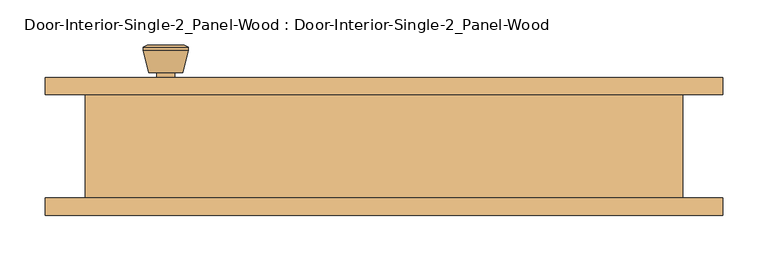
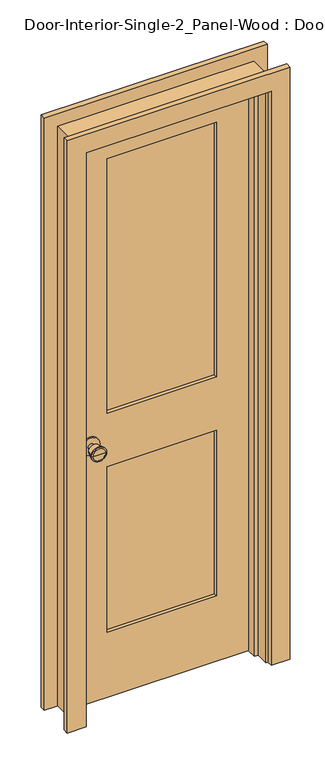
"""IFC4 building model written with IfcOpenShell, lengths in millimetres: door geometry, Door-Interior-Single-2_Panel-Wood : Door-Interior-Single-2_Panel-Wood."""

from ifc_helpers import new_model, si_unit, point, frame, frame_2d, origin, place, context, project, spatial, polyline, circle_curve, trimmed, segment, composite_curve, outline, extrude, faceted_brep, source, transform, mapped, element, save
from ifc_brep_helpers import plane_surface, cylinder_surface, revolved_surface, advanced_brep


def door_interior_single_2_panel_wood_door_interior_single_2_a051e6ed(model_context):
    return source(origin(), model_context, "Body", "SolidModel", [
        advanced_brep(
        [(-241.3, 13.05, 914.4), (-231.3, 13.05, 914.4), (-251.3, 13.05, 914.4), (-220.8241324, -35.95, 914.4), (-241.3, -35.95, 914.4), (-261.7758676, -35.95, 914.4), (-216.3, -34.1221319, 914.4), (-266.3, -34.1221319, 914.4), (-216.3, -30.6584537, 914.4), (-266.3, -30.6584537, 914.4), (-222.663764, -5.95, 914.4), (-259.936236, -5.95, 914.4), (-231.3, -5.95, 914.4), (-251.3, -5.95, 914.4)],
        [
            (0, 1),
            (1, 2, circle_curve(frame((-241.3, 13.05, 914.4), z_axis=(0.0, 1.0, 0.0), x_axis=(-1.0, 0.0, 0.0)), 10.0)),
            (2, 0),
            (2, 1, circle_curve(frame((-241.3, 13.05, 914.4), z_axis=(0.0, 1.0, 0.0), x_axis=(-1.0, 0.0, 0.0)), 10.0)),
            (3, 4),
            (4, 5),
            (5, 3, circle_curve(frame((-241.3, -35.95, 914.4), z_axis=(0.0, -1.0, 0.0), x_axis=(-1.0, 0.0, 0.0)), 20.4758676)),
            (3, 5, circle_curve(frame((-241.3, -35.95, 914.4), z_axis=(0.0, -1.0, 0.0), x_axis=(-1.0, 0.0, 0.0)), 20.4758676)),
            (6, 3),
            (5, 7),
            (7, 6, circle_curve(frame((-241.3, -34.1221319, 914.4), z_axis=(0.0, -1.0, 0.0), x_axis=(-1.0, 0.0, 0.0)), 25.0)),
            (6, 7, circle_curve(frame((-241.3, -34.1221319, 914.4), z_axis=(0.0, -1.0, 0.0), x_axis=(-1.0, 0.0, 0.0)), 25.0)),
            (8, 6),
            (7, 9),
            (9, 8, circle_curve(frame((-241.3, -30.6584537, 914.4), z_axis=(0.0, -1.0, 0.0), x_axis=(-1.0, 0.0, 0.0)), 25.0)),
            (8, 9, circle_curve(frame((-241.3, -30.6584537, 914.4), z_axis=(0.0, -1.0, 0.0), x_axis=(-1.0, 0.0, 0.0)), 25.0)),
            (10, 8),
            (9, 11),
            (11, 10, circle_curve(frame((-241.3, -5.95, 914.4), z_axis=(0.0, -1.0, 0.0), x_axis=(-1.0, 0.0, 0.0)), 18.636236)),
            (10, 11, circle_curve(frame((-241.3, -5.95, 914.4), z_axis=(0.0, -1.0, 0.0), x_axis=(-1.0, 0.0, 0.0)), 18.636236)),
            (12, 10),
            (11, 13),
            (13, 12, circle_curve(frame((-241.3, -5.95, 914.4), z_axis=(0.0, -1.0, 0.0), x_axis=(-1.0, 0.0, 0.0)), 10.0)),
            (12, 13, circle_curve(frame((-241.3, -5.95, 914.4), z_axis=(0.0, -1.0, 0.0), x_axis=(-1.0, 0.0, 0.0)), 10.0)),
            (1, 12),
            (13, 2),
        ],
        [
            plane_surface(frame((-241.3, 13.05, 914.4), z_axis=(0.0, 1.0, 0.0), x_axis=(-1.0, 0.0, 0.0))),
            plane_surface(frame((-241.3, -35.95, 914.4), z_axis=(0.0, -1.0, 0.0), x_axis=(-1.0, 0.0, 0.0))),
            revolved_surface(polyline([(-261.7758676, -35.95, 914.4), (-266.3, -34.1221319, 914.4)]), (-241.3, 13.05, 914.4), (0.0, 1.0, 0.0)),
            cylinder_surface(frame((-241.3, 13.05, 914.4), z_axis=(0.0, 1.0, 0.0), x_axis=(-1.0, 0.0, 0.0)), 25.0),
            revolved_surface(polyline([(-266.3, -30.6584537, 914.4), (-259.936236, -5.95, 914.4)]), (-241.3, 13.05, 914.4), (0.0, 1.0, 0.0)),
            plane_surface(frame((-241.3, -5.95, 914.4), z_axis=(0.0, 1.0, 0.0), x_axis=(-1.0, 0.0, 0.0))),
            cylinder_surface(frame((-241.3, 13.05, 914.4), z_axis=(0.0, 1.0, 0.0), x_axis=(-1.0, 0.0, 0.0)), 10.0),
        ],
        [
            (0, [[1, 2, 3]]),
            (0, [[-3, 4, -1]]),
            (1, [[5, 6, 7]]),
            (1, [[-6, -5, 8]]),
            (2, [[9, -7, 10, 11]]),
            (2, [[-10, -8, -9, 12]]),
            (3, [[13, -11, 14, 15]]),
            (3, [[-14, -12, -13, 16]]),
            (4, [[17, -15, 18, 19]]),
            (4, [[-18, -16, -17, 20]]),
            (5, [[21, -19, 22, 23]]),
            (5, [[-22, -20, -21, 24]]),
            (6, [[25, -23, 26, -2]]),
            (6, [[-26, -24, -25, -4]]),
        ],
    ),
        extrude(outline(composite_curve([segment(trimmed(circle_curve(frame_2d((914.4, -241.3)), 30.0), [point((914.4, -271.3))], [point((914.4, -211.3))], False, "CARTESIAN"), True, "CONTINUOUS"), segment(trimmed(circle_curve(frame_2d((914.4, -241.3)), 30.0), [point((914.4, -211.3))], [point((914.4, -271.3))], False, "CARTESIAN"), True, "CONTINUOUS")], self_intersect=False)), frame((0.0, 13.05, 0.0), z_axis=(0.0, 1.0, 0.0), x_axis=(0.0, 0.0, 1.0)), (0.0, 0.0, 1.0), 6.0),
        advanced_brep(
        [(-241.3, 59.975, 914.4), (-251.3, 59.975, 914.4), (-231.3, 59.975, 914.4), (-220.8241324, 108.975, 914.4), (-261.7758676, 108.975, 914.4), (-241.3, 108.975, 914.4), (-216.3, 107.1471319, 914.4), (-266.3, 107.1471319, 914.4), (-216.3, 103.6834537, 914.4), (-266.3, 103.6834537, 914.4), (-222.663764, 78.975, 914.4), (-259.936236, 78.975, 914.4), (-231.3, 78.975, 914.4), (-251.3, 78.975, 914.4)],
        [
            (0, 1),
            (1, 2, circle_curve(frame((-241.3, 59.975, 914.4), z_axis=(0.0, -1.0, 0.0), x_axis=(-1.0, 0.0, 0.0)), 10.0)),
            (2, 0),
            (2, 1, circle_curve(frame((-241.3, 59.975, 914.4), z_axis=(0.0, -1.0, 0.0), x_axis=(-1.0, 0.0, 0.0)), 10.0)),
            (3, 4, circle_curve(frame((-241.3, 108.975, 914.4), z_axis=(0.0, 1.0, 0.0), x_axis=(-1.0, 0.0, 0.0)), 20.4758676)),
            (4, 5),
            (5, 3),
            (4, 3, circle_curve(frame((-241.3, 108.975, 914.4), z_axis=(0.0, 1.0, 0.0), x_axis=(-1.0, 0.0, 0.0)), 20.4758676)),
            (6, 7, circle_curve(frame((-241.3, 107.1471319, 914.4), z_axis=(0.0, 1.0, 0.0), x_axis=(-1.0, 0.0, 0.0)), 25.0)),
            (7, 4),
            (3, 6),
            (7, 6, circle_curve(frame((-241.3, 107.1471319, 914.4), z_axis=(0.0, 1.0, 0.0), x_axis=(-1.0, 0.0, 0.0)), 25.0)),
            (8, 9, circle_curve(frame((-241.3, 103.6834537, 914.4), z_axis=(0.0, 1.0, 0.0), x_axis=(-1.0, 0.0, 0.0)), 25.0)),
            (9, 7),
            (6, 8),
            (9, 8, circle_curve(frame((-241.3, 103.6834537, 914.4), z_axis=(0.0, 1.0, 0.0), x_axis=(-1.0, 0.0, 0.0)), 25.0)),
            (10, 11, circle_curve(frame((-241.3, 78.975, 914.4), z_axis=(0.0, 1.0, 0.0), x_axis=(-1.0, 0.0, 0.0)), 18.636236)),
            (11, 9),
            (8, 10),
            (11, 10, circle_curve(frame((-241.3, 78.975, 914.4), z_axis=(0.0, 1.0, 0.0), x_axis=(-1.0, 0.0, 0.0)), 18.636236)),
            (12, 13, circle_curve(frame((-241.3, 78.975, 914.4), z_axis=(0.0, 1.0, 0.0), x_axis=(-1.0, 0.0, 0.0)), 10.0)),
            (13, 11),
            (10, 12),
            (13, 12, circle_curve(frame((-241.3, 78.975, 914.4), z_axis=(0.0, 1.0, 0.0), x_axis=(-1.0, 0.0, 0.0)), 10.0)),
            (1, 13),
            (12, 2),
        ],
        [
            plane_surface(frame((-241.3, 59.975, 914.4), z_axis=(0.0, -1.0, 0.0), x_axis=(-1.0, 0.0, 0.0))),
            plane_surface(frame((-241.3, 108.975, 914.4), z_axis=(0.0, 1.0, 0.0), x_axis=(-1.0, 0.0, 0.0))),
            revolved_surface(polyline([(-261.7758676, 108.975, 914.4), (-266.3, 107.1471319, 914.4)]), (-241.3, 59.975, 914.4), (0.0, -1.0, 0.0)),
            cylinder_surface(frame((-241.3, 59.975, 914.4), z_axis=(0.0, -1.0, 0.0), x_axis=(-1.0, 0.0, 0.0)), 25.0),
            revolved_surface(polyline([(-266.3, 103.6834537, 914.4), (-259.936236, 78.975, 914.4)]), (-241.3, 59.975, 914.4), (0.0, -1.0, 0.0)),
            plane_surface(frame((-241.3, 78.975, 914.4), z_axis=(0.0, -1.0, 0.0), x_axis=(-1.0, 0.0, 0.0))),
            cylinder_surface(frame((-241.3, 59.975, 914.4), z_axis=(0.0, -1.0, 0.0), x_axis=(-1.0, 0.0, 0.0)), 10.0),
        ],
        [
            (0, [[1, 2, 3]]),
            (0, [[-3, 4, -1]]),
            (1, [[5, 6, 7]]),
            (1, [[8, -7, -6]]),
            (2, [[9, 10, -5, 11]]),
            (2, [[12, -11, -8, -10]]),
            (3, [[13, 14, -9, 15]]),
            (3, [[16, -15, -12, -14]]),
            (4, [[17, 18, -13, 19]]),
            (4, [[20, -19, -16, -18]]),
            (5, [[21, 22, -17, 23]]),
            (5, [[24, -23, -20, -22]]),
            (6, [[-2, 25, -21, 26]]),
            (6, [[-4, -26, -24, -25]]),
        ],
    ),
        extrude(outline(composite_curve([segment(trimmed(circle_curve(frame_2d((914.4, -241.3)), 30.0), [point((914.4, -271.3))], [point((914.4, -211.3))], False, "CARTESIAN"), True, "CONTINUOUS"), segment(trimmed(circle_curve(frame_2d((914.4, -241.3)), 30.0), [point((914.4, -211.3))], [point((914.4, -271.3))], False, "CARTESIAN"), True, "CONTINUOUS")], self_intersect=False)), frame((0.0, 53.975, 0.0), z_axis=(0.0, 1.0, 0.0), x_axis=(0.0, 0.0, 1.0)), (0.0, 0.0, 1.0), 6.0),
        faceted_brep([(330.2, 53.975, 0.0), (330.2, -60.325, 0.0), (304.8, -60.325, 0.0), (304.8, -15.875, 0.0), (292.1, -15.875, 0.0), (292.1, 19.05, 0.0), (304.8, 19.05, 0.0), (304.8, 53.975, 0.0), (330.2, 53.975, 2057.4), (330.2, -60.325, 2057.4), (-330.2, -60.325, 2057.4), (-330.2, -60.325, 0.0), (-304.8, -60.325, 0.0), (-304.8, -60.325, 2032.0), (304.8, -60.325, 2032.0), (304.8, -15.875, 2032.0), (-304.8, -15.875, 2032.0), (-304.8, -15.875, 0.0), (-292.1, -15.875, 0.0), (-292.1, -15.875, 2019.3), (292.1, -15.875, 2019.3), (292.1, 19.05, 2019.3), (-292.1, 19.05, 2019.3), (-292.1, 19.05, 0.0), (-304.8, 19.05, 0.0), (-304.8, 19.05, 2032.0), (304.8, 19.05, 2032.0), (304.8, 53.975, 2032.0), (-304.8, 53.975, 2032.0), (-304.8, 53.975, 0.0), (-330.2, 53.975, 0.0), (-330.2, 53.975, 2057.4)], [[[0, 1, 2, 3, 4, 5, 6, 7]], [[1, 0, 8, 9]], [[2, 1, 9, 10, 11, 12, 13, 14]], [[3, 2, 14, 15]], [[4, 3, 15, 16, 17, 18, 19, 20]], [[5, 4, 20, 21]], [[6, 5, 21, 22, 23, 24, 25, 26]], [[7, 6, 26, 27]], [[0, 7, 27, 28, 29, 30, 31, 8]], [[9, 8, 31, 10]], [[15, 14, 13, 16]], [[21, 20, 19, 22]], [[27, 26, 25, 28]], [[30, 29, 24, 23, 18, 17, 12, 11]], [[10, 31, 30, 11]], [[16, 13, 12, 17]], [[22, 19, 18, 23]], [[28, 25, 24, 29]]]),
        extrude(outline(polyline([(2032.0, -304.8), (0.0, -304.8), (0.0, 304.8), (2032.0, 304.8), (2032.0, -304.8)]), holes=[polyline([(1912.9375, -184.15), (1912.9375, 184.15), (1009.65, 184.15), (1009.65, -184.15), (1912.9375, -184.15)]), polyline([(819.15, -184.15), (819.15, 184.15), (231.775, 184.15), (231.775, -184.15), (819.15, -184.15)])]), frame((0.0, 19.05, 0.0), z_axis=(0.0, 1.0, 0.0), x_axis=(0.0, 0.0, 1.0)), (0.0, 0.0, 1.0), 34.925),
        extrude(outline(polyline([(184.15, 30.6916667), (-184.15, 30.6916667), (-184.15, 42.3333333), (184.15, 42.3333333), (184.15, 30.6916667)])), frame((0.0, 0.0, 1009.65), z_axis=(0.0, 0.0, 1.0), x_axis=(1.0, 0.0, 0.0)), (0.0, 0.0, 1.0), 903.2875),
        extrude(outline(polyline([(184.15, 30.6916667), (-184.15, 30.6916667), (-184.15, 42.3333333), (184.15, 42.3333333), (184.15, 30.6916667)])), frame((0.0, 0.0, 231.775), z_axis=(0.0, 0.0, 1.0), x_axis=(1.0, 0.0, 0.0)), (0.0, 0.0, 1.0), 587.375),
        extrude(outline(polyline([(0.0, 311.15), (0.0, 374.65), (2101.85, 374.65), (2101.85, -374.65), (0.0, -374.65), (0.0, -311.15), (2038.35, -311.15), (2038.35, 311.15), (0.0, 311.15)])), frame((0.0, 53.975, 0.0), z_axis=(0.0, 1.0, 0.0), x_axis=(0.0, 0.0, 1.0)), (0.0, 0.0, 1.0), 19.05),
        extrude(outline(polyline([(0.0, 311.15), (0.0, 374.65), (2101.85, 374.65), (2101.85, -374.65), (0.0, -374.65), (0.0, -311.15), (2038.35, -311.15), (2038.35, 311.15), (0.0, 311.15)])), frame((0.0, -79.375, 0.0), z_axis=(0.0, 1.0, 0.0), x_axis=(0.0, 0.0, 1.0)), (0.0, 0.0, 1.0), 19.05),
    ])


if __name__ == "__main__":
    model = new_model("IFC4")
    model_context = context("Model", 3, world=origin())
    ifc_project = project(units=[si_unit("LENGTHUNIT", "METRE", prefix="MILLI")], contexts=[model_context])
    site = spatial("IfcSite", under=ifc_project)
    building = spatial("IfcBuilding", under=site)
    placement = place(None, origin())
    door_interior_single_2_panel_wood_door_interior_single_2_shape = door_interior_single_2_panel_wood_door_interior_single_2_a051e6ed(model_context)
    element("IfcDoor", 1, ObjectType="Door-Interior-Single-2_Panel-Wood : Door-Interior-Single-2_Panel-Wood", at=placement, inside=building, context=model_context, shape_type="MappedRepresentation", body=[
        mapped(door_interior_single_2_panel_wood_door_interior_single_2_shape, transform((0.0, 0.0, 0.0), x_axis=(1.0, 0.0, 0.0), y_axis=(0.0, 1.0, 0.0), z_axis=(0.0, 0.0, 1.0))),
    ])
    save(model, "model.ifc")

# Revit data of these elements
# Type "Door-Interior-Single-2_Panel-Wood : Door-Interior-Single-2_Panel-Wood"
#   Type Mark = "12"
#   Assembly Code = "C1020300"
#   Analytic Construction = "Wooden"
#   Top Rail = 0' - 4 11/16"
#   Thickness = 0' - 1 3/8"
#   Thermal Resistance (R) = 2.5876 (h·ft²·°F)/BTU
#   Swing Angle [instance default] = 90.00°
#   Stiles = 0' - 4 3/4"
#   Rough Width = 2' - 2"
#   Rough Height = 6' - 9"
#   Lock Rail = 0' - 7 1/2"
#   Height = 6' - 8"
#   Width = 2' - 0"
#   Heat Transfer Coefficient (U) = 0.3865 BTU/(h·ft²·°F)
#   Bottom Rail = 0' - 9 1/8"
#   Trim Material = Cherry
#   Panel Material = Cherry
#   Frame Material = Cherry
#   Door Handle Material = Aluminum
#   Visual Light Transmittance = 0
#   Solar Heat Gain Coefficient = 0
#   Wall Closure = (empty or 0)
#   Function = (empty or 0)
# Element 1 (IfcDoor, "Door-Interior-Single-2_Panel-Wood : Door-Interior-Single-2_Panel-Wood")
#   Materials on its faces: "Cherry", "Aluminum"
# Materials
#   "Cherry": class "Wood", colour RGB 226 177 128, transparency 0, Description = "Prunus Serotina", Cost = 0
#   "Aluminum": class "Metal", colour RGB 247 247 247, transparency 0, Description = "Aluminum 6061", Cost = 0
